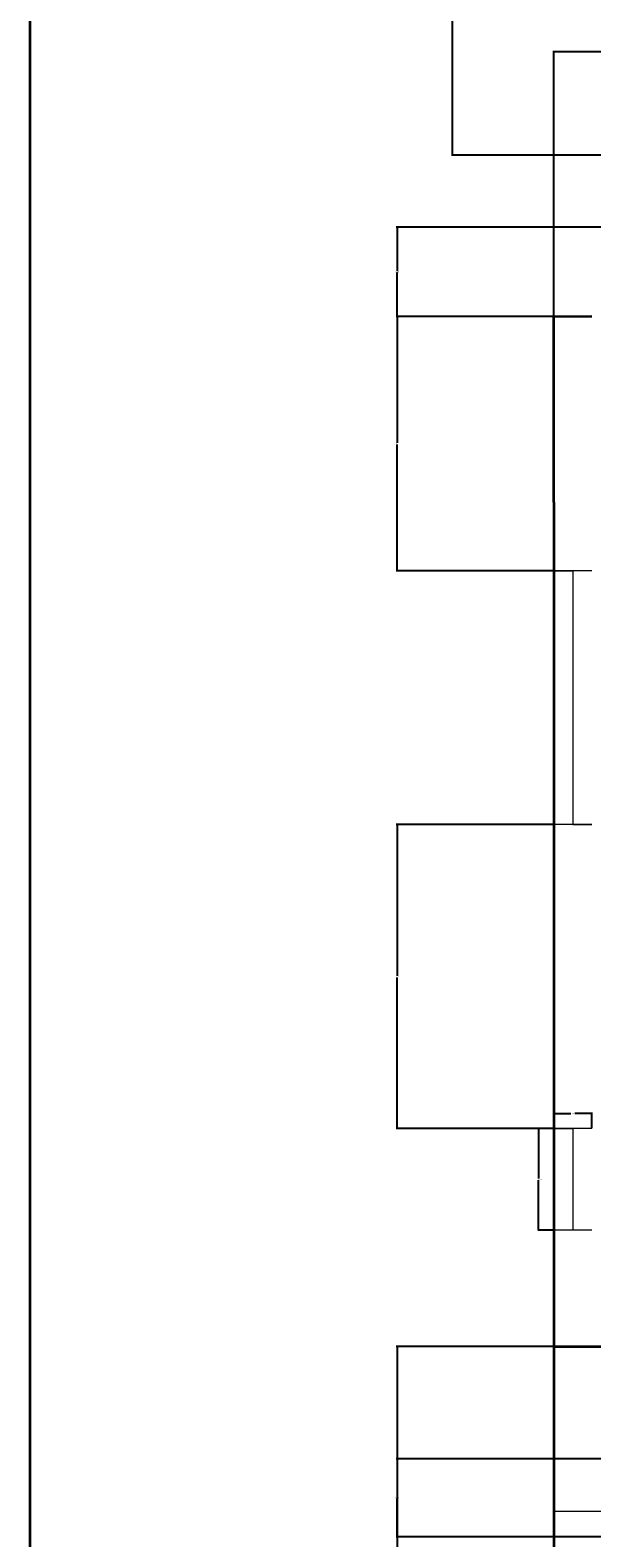
# Model space of a CAD drawing. Units: inches. Extents: x 1854 to 2495, y 1460 to 2772.
# Tile 7 of 12: x 1854 to 1987, y 1958 to 2314. Entities that reach past the tile are written whole.
import ezdxf

# ---------------------------------------------------------------- set-up
doc = ezdxf.new("R2010")
doc.units = ezdxf.units.IN
for name, color, linetype, lineweight in [('A-ANNO-DIMS', 2, 'Continuous', 18), ('A-ANNO-TTLB', 7, 'Continuous', 35), ('A-FLOR-STRS', 7, 'Continuous', 18), ('A-GLAZ', 4, 'Continuous', 18), ('A-WALL', 7, 'Continuous', 35)]:
    doc.layers.add(name, color=color, linetype=linetype, lineweight=lineweight)
doc.styles.get("Standard").update_dxf_attribs({"font": 'arial.ttf'})
doc.dimstyles.get("Standard").update_dxf_attribs({"dimtxt": 0.18, "dimasz": 0.18, "dimexe": 0.18, "dimexo": 0.0625, "dimgap": 0.09, "dimtad": 0, "dimtih": 1, "dimtoh": 1, "dimdec": 4, "dimzin": 0, "dimdsep": 46, "dimtxsty": 'Standard', "dimcen": 0.09, "dimadec": 0, "dimazin": 0, "dimtfac": 1, "dimtdec": 4, "dimtofl": 0, "dimtmove": 0, "dimatfit": 3, "dimfxl": 1, "dimtolj": 1, "dimtzin": 0, "dimarcsym": 0})

# ---------------------------------------------------------------- blocks, each defined once
blk = doc.blocks.new('WINDOW-60IN')
for p, q in [((0, 9), (0, 0)), ((60, 4.5), (60, 9)), ((60, 9), (60, 0)), ((0, 0), (0, 4.5)), ((0, 4.5), (60, 4.5))]:
    blk.add_line(p, q)
blk = doc.blocks.new('WINDOW-VENT-24IN')
for p, q in [((9, 24), (0, 24)), ((4.5, 24), (4.5, 0)), ((9, 0), (0, 0))]:
    blk.add_line(p, q)
blk = doc.blocks.new('*D35')
at = {"layer": 'A-ANNO-DIMS', "color": 0, "lineweight": -2, "transparency": 16777216}
for p, q in [((1977.92, 2054.53), (1974.2, 2054.53)), ((1974.38, 2054.35), (1974.38, 2042.71)), ((1974.38, 2030.71), (1974.38, 2042.35)), ((1977.92, 2030.53), (1974.2, 2030.53))]:
    blk.add_line(p, q, dxfattribs=at)
at = {"layer": 'A-ANNO-DIMS', "color": 0, "transparency": 16777216}
for points in [[(1974.35, 2054.35), (1974.41, 2054.35), (1974.38, 2054.53)], [(1974.35, 2030.71), (1974.41, 2030.71), (1974.38, 2030.53)]]:
    blk.add_solid(points, dxfattribs=at)
at = {"layer": 'Defpoints', "color": 0, "transparency": 16777216}
for p in [(1974.38, 2054.53), (1977.98, 2054.53), (1977.98, 2030.53)]:
    blk.add_point(p, dxfattribs=at)
at = {"layer": 'A-ANNO-DIMS', "color": 0, "transparency": 16777216, "insert": (1974.38, 2042.53), "char_height": 0.18, "attachment_point": 5}
blk.add_mtext('\\A1;EXT. VENT 24 TYP.', dxfattribs=at)
blk = doc.blocks.new('*D36')
at = {"layer": 'A-ANNO-DIMS', "color": 0, "lineweight": -2, "transparency": 16777216}
for p, q in [((1977.98, 2054.59), (1977.98, 2058.31)), ((1978.16, 2058.13), (1982.02, 2058.13)), ((1986.8, 2058.13), (1982.94, 2058.13)), ((1986.98, 2054.59), (1986.98, 2058.31))]:
    blk.add_line(p, q, dxfattribs=at)
at = {"layer": 'A-ANNO-DIMS', "color": 0, "transparency": 16777216}
for points in [[(1978.16, 2058.16), (1978.16, 2058.1), (1977.98, 2058.13)], [(1986.8, 2058.16), (1986.8, 2058.1), (1986.98, 2058.13)]]:
    blk.add_solid(points, dxfattribs=at)
at = {"layer": 'Defpoints', "color": 0, "transparency": 16777216}
for p in [(1986.98, 2058.13), (1977.98, 2054.53), (1986.98, 2054.53)]:
    blk.add_point(p, dxfattribs=at)
at = {"layer": 'A-ANNO-DIMS', "color": 0, "transparency": 16777216, "insert": (1982.48, 2058.13), "char_height": 0.18, "attachment_point": 5}
blk.add_mtext('\\A1;9 TYP.', dxfattribs=at)
blk = doc.blocks.new('*D49')
at = {"layer": 'A-ANNO-DIMS', "color": 0, "lineweight": -2, "transparency": 16777216}
for p, q in [((1977.98, 2246.51), (1977.98, 2309.27)), ((1978.16, 2309.09), (2179.19, 2309.09)), ((2380.8, 2309.09), (2179.77, 2309.09)), ((2380.98, 2272.11), (2380.98, 2309.27))]:
    blk.add_line(p, q, dxfattribs=at)
at = {"layer": 'A-ANNO-DIMS', "color": 0, "transparency": 16777216}
for points in [[(1978.16, 2309.12), (1978.16, 2309.06), (1977.98, 2309.09)], [(2380.8, 2309.12), (2380.8, 2309.06), (2380.98, 2309.09)]]:
    blk.add_solid(points, dxfattribs=at)
at = {"layer": 'Defpoints', "color": 0, "transparency": 16777216}
for p in [(2380.98, 2309.09), (2380.98, 2272.04), (1977.98, 2246.45)]:
    blk.add_point(p, dxfattribs=at)
at = {"layer": 'A-ANNO-DIMS', "color": 0, "transparency": 16777216, "insert": (2179.48, 2309.09), "char_height": 0.18, "attachment_point": 5}
blk.add_mtext('\\A1;403', dxfattribs=at)
blk = doc.blocks.new('*D54')
at = {"layer": 'A-ANNO-DIMS', "color": 0, "lineweight": -2, "transparency": 16777216}
for p, q in [((1977.92, 2003.04), (1940.75, 2003.04)), ((1940.93, 2002.86), (1940.93, 1925.23)), ((1940.93, 1847.22), (1940.93, 1924.86)), ((1977.92, 1847.04), (1940.75, 1847.04))]:
    blk.add_line(p, q, dxfattribs=at)
at = {"layer": 'A-ANNO-DIMS', "color": 0, "transparency": 16777216}
for points in [[(1940.9, 2002.86), (1940.96, 2002.86), (1940.93, 2003.04)], [(1940.9, 1847.22), (1940.96, 1847.22), (1940.93, 1847.04)]]:
    blk.add_solid(points, dxfattribs=at)
at = {"layer": 'Defpoints', "color": 0, "transparency": 16777216}
for p in [(1940.93, 2003.04), (1977.98, 2003.04), (1977.98, 1847.04)]:
    blk.add_point(p, dxfattribs=at)
at = {"layer": 'A-ANNO-DIMS', "color": 0, "transparency": 16777216, "insert": (1940.93, 1925.04), "char_height": 0.18, "attachment_point": 5}
blk.add_mtext('\\A1;156', dxfattribs=at)
blk = doc.blocks.new('*D55')
at = {"layer": 'A-ANNO-DIMS', "color": 0, "lineweight": -2, "transparency": 16777216}
for p, q in [((1977.92, 2126.37), (1940.75, 2126.37)), ((1940.93, 2126.19), (1940.93, 2090.63)), ((1940.93, 2054.71), (1940.93, 2090.27)), ((1977.92, 2054.53), (1940.75, 2054.53))]:
    blk.add_line(p, q, dxfattribs=at)
at = {"layer": 'A-ANNO-DIMS', "color": 0, "transparency": 16777216}
for points in [[(1940.9, 2126.19), (1940.96, 2126.19), (1940.93, 2126.37)], [(1940.9, 2054.71), (1940.96, 2054.71), (1940.93, 2054.53)]]:
    blk.add_solid(points, dxfattribs=at)
at = {"layer": 'Defpoints', "color": 0, "transparency": 16777216}
for p in [(1940.93, 2126.37), (1977.98, 2126.37), (1977.98, 2054.53)]:
    blk.add_point(p, dxfattribs=at)
at = {"layer": 'A-ANNO-DIMS', "color": 0, "transparency": 16777216, "insert": (1940.93, 2090.45), "char_height": 0.18, "attachment_point": 5}
blk.add_mtext('\\A1;71.84', dxfattribs=at)
blk = doc.blocks.new('*D56')
at = {"layer": 'A-ANNO-DIMS', "color": 0, "lineweight": -2, "transparency": 16777216}
for p, q in [((1977.92, 2246.45), (1940.75, 2246.45)), ((1940.93, 2246.27), (1940.93, 2216.59)), ((1940.93, 2186.55), (1940.93, 2216.23)), ((1977.92, 2186.37), (1940.75, 2186.37))]:
    blk.add_line(p, q, dxfattribs=at)
at = {"layer": 'A-ANNO-DIMS', "color": 0, "transparency": 16777216}
for points in [[(1940.9, 2246.27), (1940.96, 2246.27), (1940.93, 2246.45)], [(1940.9, 2186.55), (1940.96, 2186.55), (1940.93, 2186.37)]]:
    blk.add_solid(points, dxfattribs=at)
at = {"layer": 'Defpoints', "color": 0, "transparency": 16777216}
for p in [(1940.93, 2246.45), (1977.98, 2246.45), (1977.98, 2186.37)]:
    blk.add_point(p, dxfattribs=at)
at = {"layer": 'A-ANNO-DIMS', "color": 0, "transparency": 16777216, "insert": (1940.93, 2216.41), "char_height": 0.18, "attachment_point": 5}
blk.add_mtext('\\A1;60.08', dxfattribs=at)
blk = doc.blocks.new('*D57')
at = {"layer": 'A-ANNO-DIMS', "color": 0, "lineweight": -2, "transparency": 16777216}
for p, q in [((2105.42, 2267.54), (1940.75, 2267.54)), ((1940.93, 2267.36), (1940.93, 2257.18)), ((1940.93, 2246.63), (1940.93, 2256.82)), ((1977.92, 2246.45), (1940.75, 2246.45))]:
    blk.add_line(p, q, dxfattribs=at)
at = {"layer": 'A-ANNO-DIMS', "color": 0, "transparency": 16777216}
for points in [[(1940.9, 2267.36), (1940.96, 2267.36), (1940.93, 2267.54)], [(1940.9, 2246.63), (1940.96, 2246.63), (1940.93, 2246.45)]]:
    blk.add_solid(points, dxfattribs=at)
at = {"layer": 'Defpoints', "color": 0, "transparency": 16777216}
for p in [(1940.93, 2267.54), (2105.48, 2267.54), (1977.98, 2246.45)]:
    blk.add_point(p, dxfattribs=at)
at = {"layer": 'A-ANNO-DIMS', "color": 0, "transparency": 16777216, "insert": (1940.93, 2257), "char_height": 0.18, "attachment_point": 5}
blk.add_mtext('\\A1;21.095', dxfattribs=at)
blk = doc.blocks.new('*D61')
at = {"layer": 'A-ANNO-DIMS', "color": 0, "lineweight": -2, "transparency": 16777216}
for p, q in [((1977.98, 1847.11), (1977.98, 2309.27)), ((1978.16, 2309.09), (1997.26, 2309.09)), ((2016.8, 2309.09), (1997.7, 2309.09)), ((2016.98, 1847.11), (2016.98, 2309.27))]:
    blk.add_line(p, q, dxfattribs=at)
at = {"layer": 'A-ANNO-DIMS', "color": 0, "transparency": 16777216}
for points in [[(1978.16, 2309.12), (1978.16, 2309.06), (1977.98, 2309.09)], [(2016.8, 2309.12), (2016.8, 2309.06), (2016.98, 2309.09)]]:
    blk.add_solid(points, dxfattribs=at)
at = {"layer": 'Defpoints', "color": 0, "transparency": 16777216}
for p in [(2016.98, 2309.09), (1977.98, 1847.04), (2016.98, 1847.04)]:
    blk.add_point(p, dxfattribs=at)
at = {"layer": 'A-ANNO-DIMS', "color": 0, "transparency": 16777216, "insert": (1997.48, 2309.09), "char_height": 0.18, "attachment_point": 5}
blk.add_mtext('\\A1;39', dxfattribs=at)
blk = doc.blocks.new('*D63')
at = {"layer": 'A-ANNO-DIMS', "color": 0, "lineweight": -2, "transparency": 16777216}
for p, q in [((1977.98, 2246.39), (1977.98, 1503.44)), ((2007.19, 2246.48), (2007.19, 1503.44)), ((1978.16, 1503.62), (1992.21, 1503.62)), ((2007.01, 1503.62), (1992.96, 1503.62))]:
    blk.add_line(p, q, dxfattribs=at)
at = {"layer": 'A-ANNO-DIMS', "color": 0, "transparency": 16777216}
for points in [[(1978.16, 1503.65), (1978.16, 1503.59), (1977.98, 1503.62)], [(2007.01, 1503.65), (2007.01, 1503.59), (2007.19, 1503.62)]]:
    blk.add_solid(points, dxfattribs=at)
at = {"layer": 'Defpoints', "color": 0, "transparency": 16777216}
for p in [(1977.98, 2246.45), (2007.19, 2246.54), (2007.19, 1503.62)]:
    blk.add_point(p, dxfattribs=at)
at = {"layer": 'A-ANNO-DIMS', "color": 0, "transparency": 16777216, "insert": (1992.59, 1503.62), "char_height": 0.18, "attachment_point": 5}
blk.add_mtext('\\A1;29.21', dxfattribs=at)
blk = doc.blocks.new('*D68')
at = {"layer": 'A-ANNO-DIMS', "color": 0, "lineweight": -2, "transparency": 16777216}
for p, q in [((2371.92, 1976.49), (1940.75, 1976.49)), ((1940.93, 1976.31), (1940.93, 1967.45)), ((1940.93, 1958.22), (1940.93, 1967.08)), ((2371.92, 1958.04), (1940.75, 1958.04))]:
    blk.add_line(p, q, dxfattribs=at)
at = {"layer": 'A-ANNO-DIMS', "color": 0, "transparency": 16777216}
for points in [[(1940.9, 1976.31), (1940.96, 1976.31), (1940.93, 1976.49)], [(1940.9, 1958.22), (1940.96, 1958.22), (1940.93, 1958.04)]]:
    blk.add_solid(points, dxfattribs=at)
at = {"layer": 'Defpoints', "color": 0, "transparency": 16777216}
for p in [(2371.98, 1976.49), (1940.93, 1958.04), (2371.98, 1958.04)]:
    blk.add_point(p, dxfattribs=at)
at = {"layer": 'A-ANNO-DIMS', "color": 0, "transparency": 16777216, "insert": (1940.93, 1967.27), "char_height": 0.18, "attachment_point": 5}
blk.add_mtext('\\A1;18.442', dxfattribs=at)
blk = doc.blocks.new('*D74')
at = {"layer": 'A-ANNO-DIMS', "color": 0, "lineweight": -2, "transparency": 16777216}
for p, q in [((1953.98, 2372.03), (1953.98, 2284.46)), ((2404.98, 2372.03), (2404.98, 2284.46)), ((1954.16, 2284.64), (2179.21, 2284.64)), ((2404.8, 2284.64), (2179.76, 2284.64))]:
    blk.add_line(p, q, dxfattribs=at)
at = {"layer": 'A-ANNO-DIMS', "color": 0, "transparency": 16777216}
for points in [[(1954.16, 2284.67), (1954.16, 2284.61), (1953.98, 2284.64)], [(2404.8, 2284.67), (2404.8, 2284.61), (2404.98, 2284.64)]]:
    blk.add_solid(points, dxfattribs=at)
at = {"layer": 'Defpoints', "color": 0, "transparency": 16777216}
for p in [(1953.98, 2372.09), (2404.98, 2372.09), (2404.98, 2284.64)]:
    blk.add_point(p, dxfattribs=at)
at = {"layer": 'A-ANNO-DIMS', "color": 0, "transparency": 16777216, "insert": (2179.48, 2284.64), "char_height": 0.18, "attachment_point": 5}
blk.add_mtext('\\A1;451', dxfattribs=at)

msp = doc.modelspace()

# ---------------------------------------------------------------- linework, layer by layer
at = {"layer": 'A-ANNO-TTLB'}
msp.add_lwpolyline([(1854.1764, 2772.4852), (2494.521, 2772.4852), (2494.521, 1460.4076), (1854.1764, 1460.4076)], close=True, dxfattribs=at)
at = {"layer": 'A-FLOR-STRS'}
msp.add_line((2016.9824, 1964.0449), (1977.9824, 1964.0449), dxfattribs=at)
at = {"layer": 'A-GLAZ'}
for p, q in [((1977.9824, 2054.5278), (1982.4824, 2054.5278)), ((1982.4824, 2030.5278), (1977.9824, 2030.5278))]:
    msp.add_line(p, q, dxfattribs=at)
at = {"layer": 'A-WALL'}
for p, q in [((1977.9824, 2246.45), (1986.9824, 2246.5449)), ((1977.9824, 2202.5449), (1977.9824, 2246.45)), ((1977.9824, 2202.5449), (1977.9824, 1594.5449)), ((1977.9824, 2003.0449), (2095.3698, 2003.0449))]:
    msp.add_line(p, q, dxfattribs=at)

# ---------------------------------------------------------------- block references
at = {"layer": 'A-GLAZ', "rotation": 270.0000000000002}
msp.add_blockref('WINDOW-60IN', (1977.9825, 2186.3716), dxfattribs=at)
at = {"layer": 'A-GLAZ'}
msp.add_blockref('WINDOW-VENT-24IN', (1977.982, 2030.528), dxfattribs=at)

# ---------------------------------------------------------------- dimensions: what is measured, and where the dimension line sits
at = {"layer": 'A-ANNO-DIMS'}
for base, p1, p2, override, picture, middle in [((2404.9824, 2284.6405), (1953.9824, 2372.0884), (2404.9824, 2372.0884), {"dimdec": 0, "dimlfac": 1, "dimrnd": 0, "dimzin": 0, "dimdsep": 46, "dimlunit": 2}, '*D74', (2179.4824, 2284.6405)), ((2380.9824, 2309.0949), (1977.9824, 2246.45), (2380.9824, 2272.0449), {"dimdec": 0, "dimlfac": 1, "dimrnd": 0, "dimzin": 0, "dimdsep": 46, "dimlunit": 2}, '*D49', (2179.4824, 2309.0949)), ((2016.9824, 2309.0949), (1977.9824, 1847.0449), (2016.9824, 1847.0449), {"dimdec": 0, "dimlfac": 1, "dimrnd": 0, "dimzin": 0, "dimdsep": 46, "dimlunit": 2}, '*D61', (1997.4824, 2309.0949)), ((2007.1898, 1503.6207), (1977.9824, 2246.45), (2007.1898, 2246.5449), {"dimdec": 2, "dimlfac": 1, "dimrnd": 0, "dimzin": 0, "dimdsep": 46, "dimlunit": 2}, '*D63', (1992.5861, 1503.6207))]:
    dim = msp.add_linear_dim(base=base, p1=p1, p2=p2, dimstyle='Standard', override=override, dxfattribs=at)
    dim.commit()
    dim.dimension.update_dxf_attribs({"geometry": picture, "text_midpoint": middle})
for base, p1, p2, override, picture, middle in [((1940.9324, 2267.5449), (1977.9824, 2246.45), (2105.4824, 2267.5449), {"dimdec": 3, "dimlfac": 1, "dimrnd": 0, "dimzin": 0, "dimdsep": 46, "dimlunit": 2}, '*D57', (1940.9324, 2256.9975)), ((1940.9324, 2246.45), (1977.9824, 2186.3718), (1977.9824, 2246.45), {"dimdec": 2, "dimlfac": 1, "dimrnd": 0, "dimzin": 0, "dimdsep": 46, "dimlunit": 2}, '*D56', (1940.9324, 2216.4109)), ((1940.9324, 2126.3718), (1977.9824, 2054.5278), (1977.9824, 2126.3718), {"dimdec": 2, "dimlfac": 1, "dimrnd": 0, "dimzin": 0, "dimdsep": 46, "dimlunit": 2}, '*D55', (1940.9324, 2090.4498)), ((1940.9324, 2003.0449), (1977.9824, 1847.0449), (1977.9824, 2003.0449), {"dimdec": 0, "dimlfac": 1, "dimrnd": 0, "dimzin": 0, "dimdsep": 46, "dimlunit": 2}, '*D54', (1940.9324, 1925.0449)), ((1940.93239, 1958.04492), (2371.98239, 1976.48735), (2371.98239, 1958.04492), {"dimdec": 3, "dimlfac": 1, "dimrnd": 0, "dimzin": 0, "dimdsep": 46, "dimlunit": 2}, '*D68', (1940.93239, 1967.26613))]:
    dim = msp.add_linear_dim(base=base, p1=p1, p2=p2, angle=90, dimstyle='Standard', override=override, dxfattribs=at)
    dim.commit()
    dim.dimension.update_dxf_attribs({"geometry": picture, "text_midpoint": middle})
dim = msp.add_linear_dim(base=(1986.9824, 2058.1278), p1=(1977.9824, 2054.5278), p2=(1986.9824, 2054.5278), text='<> TYP.', dimstyle='Standard', override={"dimdec": 0, "dimlfac": 1, "dimrnd": 0, "dimzin": 0, "dimdsep": 46, "dimlunit": 2}, dxfattribs=at)
dim.commit()
dim.dimension.update_dxf_attribs({"geometry": '*D36', "text_midpoint": (1982.4824, 2058.1278)})
dim = msp.add_linear_dim(base=(1974.3824, 2054.5278), p1=(1977.9824, 2030.5278), p2=(1977.9824, 2054.5278), angle=90, text='EXT. VENT <> TYP.', dimstyle='Standard', override={"dimdec": 0, "dimlfac": 1, "dimrnd": 0, "dimzin": 0, "dimdsep": 46, "dimlunit": 2}, dxfattribs=at)
dim.commit()
dim.dimension.update_dxf_attribs({"geometry": '*D35', "text_midpoint": (1974.3824, 2042.5278)})

doc.saveas('drawing.dxf')
